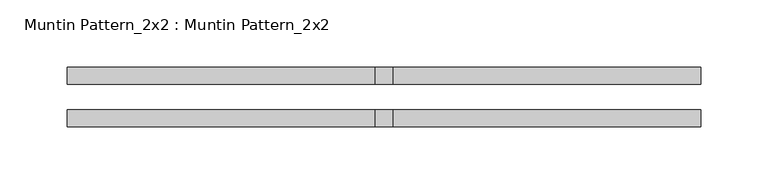
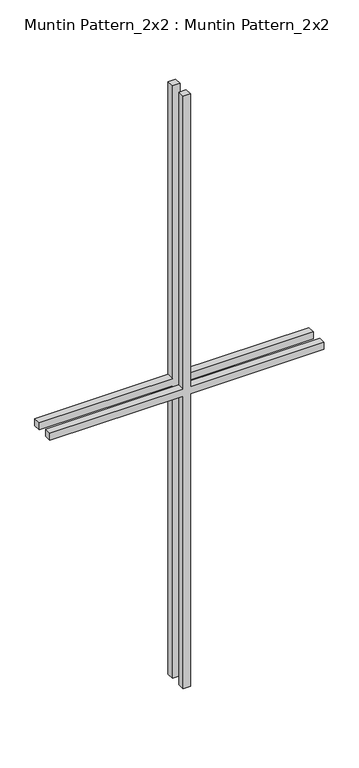
"""IFC4 building model written with IfcOpenShell, lengths in millimetres: proxy geometry, Muntin Pattern_2x2 : Muntin Pattern_2x2."""

from ifc_helpers import new_model, si_unit, frame, origin, place, context, project, spatial, polyline, outline, extrude, source, transform, mapped, element, save


def muntin_pattern_2x2_muntin_pattern_2x2_e852a7e4(model_context):
    return source(origin(), model_context, "Body", "SweptSolid", [
        extrude(outline(polyline([(546.1, -6.35), (546.1, -236.5375), (533.4, -236.5375), (533.4, -6.35), (0.0, -6.35), (0.0, 6.35), (533.4, 6.35), (533.4, 236.5375), (546.1, 236.5375), (546.1, 6.35), (1079.5, 6.35), (1079.5, -6.35), (546.1, -6.35)])), frame((0.0, -22.225, 0.0), z_axis=(0.0, 1.0, 0.0), x_axis=(0.0, 0.0, 1.0)), (0.0, 0.0, 1.0), 12.7),
        extrude(outline(polyline([(546.1, -6.35), (546.1, -236.5375), (533.4, -236.5375), (533.4, -6.35), (0.0, -6.35), (0.0, 6.35), (533.4, 6.35), (533.4, 236.5375), (546.1, 236.5375), (546.1, 6.35), (1079.5, 6.35), (1079.5, -6.35), (546.1, -6.35)])), frame((0.0, 9.525, 0.0), z_axis=(0.0, 1.0, 0.0), x_axis=(0.0, 0.0, 1.0)), (0.0, 0.0, 1.0), 12.7),
    ])


if __name__ == "__main__":
    model = new_model("IFC4")
    model_context = context("Model", 3, world=origin())
    ifc_project = project(units=[si_unit("LENGTHUNIT", "METRE", prefix="MILLI")], contexts=[model_context])
    site = spatial("IfcSite", under=ifc_project)
    building = spatial("IfcBuilding", under=site)
    placement = place(None, origin())
    muntin_pattern_2x2_muntin_pattern_2x2_shape = muntin_pattern_2x2_muntin_pattern_2x2_e852a7e4(model_context)
    element("IfcBuildingElementProxy", 1, Name="Muntin Pattern_2x2 : Muntin Pattern_2x2", ObjectType="Muntin Pattern_2x2 : Muntin Pattern_2x2", at=placement, inside=building, context=model_context, shape_type="MappedRepresentation", body=[
        mapped(muntin_pattern_2x2_muntin_pattern_2x2_shape, transform((0.0, 0.0, 0.0), x_axis=(1.0, 0.0, 0.0), y_axis=(0.0, 1.0, 0.0), z_axis=(0.0, 0.0, 1.0))),
    ])
    save(model, "model.ifc")

# Revit data of these elements
# Type "Muntin Pattern_2x2 : Muntin Pattern_2x2"
#   Width [instance default] = 4' - 0"
#   Thickness = 0' - 0 1/2"
#   Height [instance default] = 4' - 0"
#   Distance = 0' - 0 3/4"
#   Interior Material [instance default] = none
#   Exterior Material [instance default] = none
#   Default Elevation = 0
# Element 1 (IfcBuildingElementProxy, "Muntin Pattern_2x2 : Muntin Pattern_2x2")
#   Width = 1' - 6 5/8"
#   Height = 3' - 6 1/2"
#   Interior Material = Wood - Stained
#   Exterior Material = Clad - White
#   Materials on its faces: "Clad - White", "Wood - Stained"
# Materials
#   "Clad - White": class "Wood", colour RGB 242 242 238, transparency 0, Cost = 0
#   "Wood - Stained": class "Wood", colour RGB 224 178 126, transparency 0, Cost = 0
